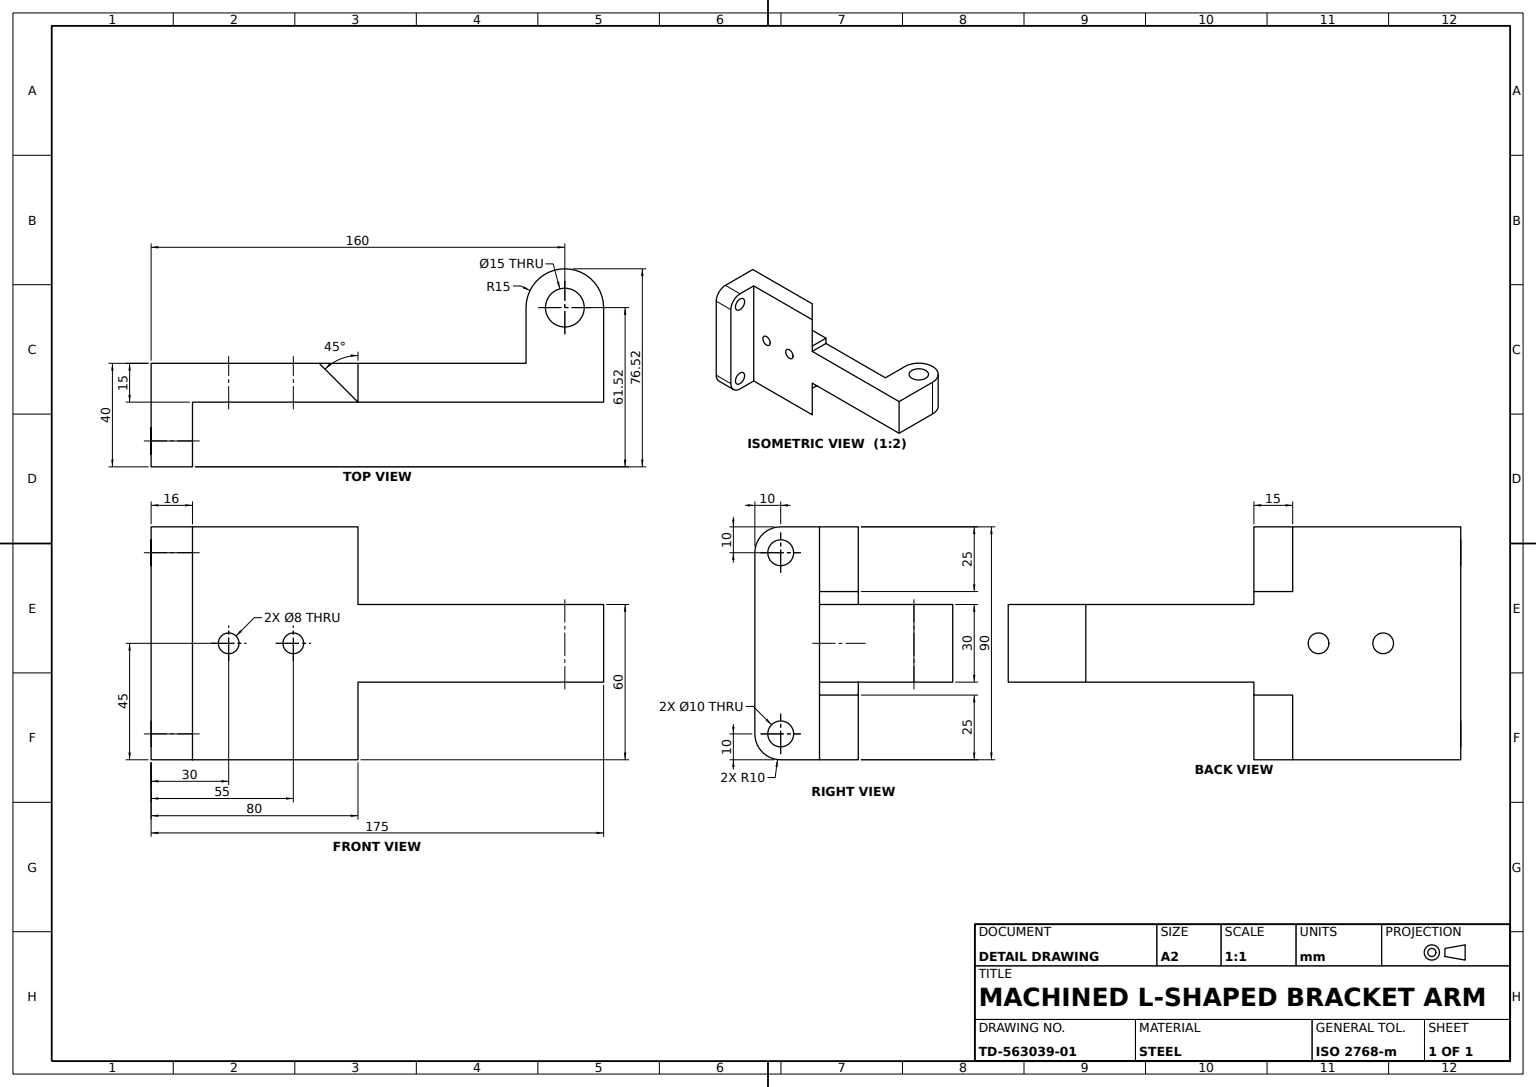
from build123d import *

# Parameters (mm, degrees)
BRACKET_BODY_DEPTH         = 90
ANGLED_CUT_DEPTH           = 25
ARM_BOSS_SKETCH_R          = 7.5
ARM_BOSS_DEPTH             = 15
CORNER_FILLETS_R10_R       = 10
CORNER_HOLES_10_DEPTH      = 202.651164925
CORNER_HOLES_10_DEPTH_BACK = 202.651164925
CORNER_HOLES_SKETCH_R      = 5
FACE_HOLES_2X_8_DEPTH      = 168.107749671
FACE_HOLES_2X_8_DEPTH_BACK = 168.107749671
FACE_HOLES_SKETCH_R        = 4


with BuildPart() as part:
    # Bracket Profile Sketch → Bracket Body (new body)
    with BuildSketch(Plane(origin=(0, 0, 0), x_dir=(1, 0, 0), z_dir=(0, 1, 0))):
        Polygon((-24, -7.5), (-24, -32.5), (-40, -32.5), (-40, 7.5), (-24, 7.5), (40, 7.5), (40, -7.5), align=None)
    extrude(amount=BRACKET_BODY_DEPTH)

    # Angled Cut Sketch → Angled Cut (cut)
    with BuildSketch(Plane(origin=(0, 90, 0), x_dir=(1, 0, 0), z_dir=(0, 1, 0))):
        Polygon((40, 7.5), (25, 7.5), (40, -7.5), align=None)
    angled_cut = extrude(amount=-ANGLED_CUT_DEPTH, mode=Mode.SUBTRACT)

    # Angled Cut Mirror: Angled Cut across plane
    add(angled_cut.mirror(Plane.ZX.offset(45)), mode=Mode.SUBTRACT)

    # Arm Boss Sketch → Arm Boss (add, symmetric)
    with BuildSketch(Plane(origin=(0, 45, 0), x_dir=(1, 0, 0), z_dir=(0, 1, 0))):
        with BuildLine():
            Line((40, -7.5), (135, -7.5))
            Line((135, -7.5), (135, 29.024905628))
            ThreePointArc((135, 29.024905628), (120, 44.024905628), (105, 29.024905628))
            Line((105, 29.024905628), (105, 7.5))
            Line((105, 7.5), (40, 7.5))
            Line((40, 7.5), (40, -7.5))
        make_face()
        with Locations(Location((120, 29.024905628, 0), (0, 0, 270))):
            Circle(ARM_BOSS_SKETCH_R, mode=Mode.SUBTRACT)
    extrude(amount=ARM_BOSS_DEPTH, both=True)

    # Corner Fillets R10
    corner_fillets_r10_edges = [part.edges().sort_by_distance(p)[0] for p in [
        (-32, 90, 32.5),
        (-32, 0, 32.5),
    ]]
    fillet(corner_fillets_r10_edges, radius=CORNER_FILLETS_R10_R)

    # Corner Holes Sketch → Corner Holes Ø10 (cut, two sides: drawn at the far end of the back side and taken through both)
    with BuildSketch(Plane.ZY.offset(40).offset(-CORNER_HOLES_10_DEPTH_BACK)):
        with Locations((22.5, 80)):
            Circle(CORNER_HOLES_SKETCH_R)
        with Locations((22.5, 10)):
            Circle(CORNER_HOLES_SKETCH_R)
    extrude(amount=CORNER_HOLES_10_DEPTH + CORNER_HOLES_10_DEPTH_BACK, mode=Mode.SUBTRACT)

    # Face Holes Sketch → Face Holes 2xØ8 (cut, two sides: drawn at the far end of the back side and taken through both)
    with BuildSketch(Plane(origin=(0, 0, -7.5), x_dir=(-1, 0, 0), z_dir=(0, 0, -1)).offset(-FACE_HOLES_2X_8_DEPTH_BACK)):
        with Locations((10, 45)):
            Circle(FACE_HOLES_SKETCH_R)
        with Locations((-15, 45)):
            Circle(FACE_HOLES_SKETCH_R)
    extrude(amount=FACE_HOLES_2X_8_DEPTH + FACE_HOLES_2X_8_DEPTH_BACK, mode=Mode.SUBTRACT)


solid = part.part
